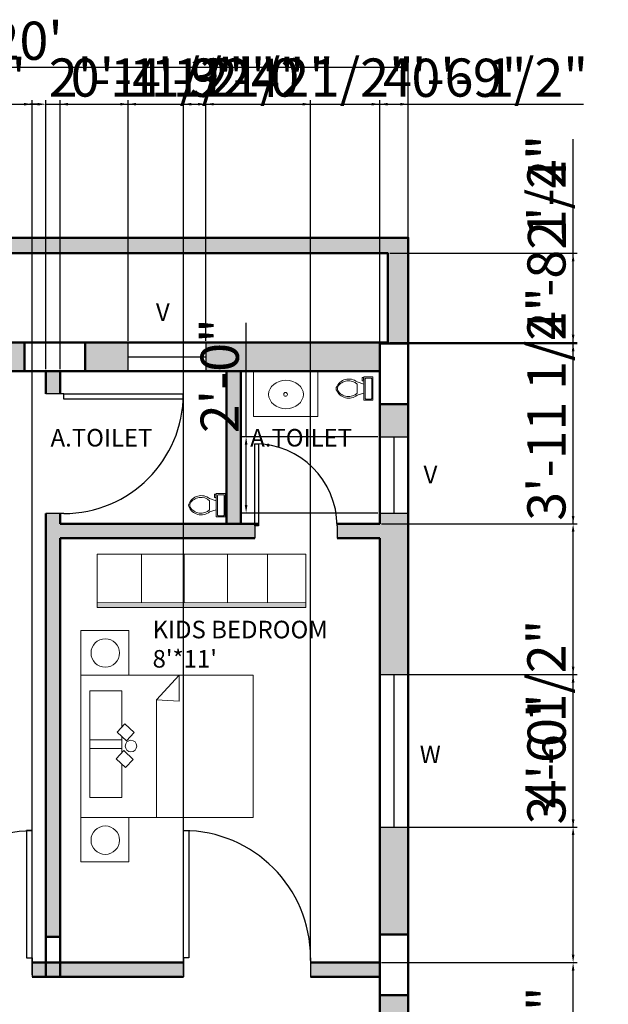
# Model space of a CAD drawing. Units: inches. Extents: x 2063 to 3370, y 2091 to 2971.
# Tile 10 of 14: x 2721 to 2906, y 2623 to 2933. Entities that reach past the tile are written whole.
import ezdxf

# ---------------------------------------------------------------- set-up
doc = ezdxf.new("R2010")
doc.units = ezdxf.units.IN
for name, color, linetype, lineweight in [('A-ANNO-DIMS', 2, 'Continuous', 18), ('A-ANNO-TEXT', 7, 'Continuous', 18), ('A-AREA-IDEN', 3, 'Continuous', 18), ('A-COLS', 7, 'Continuous', 50), ('A-DOOR', 4, 'Continuous', 25), ('A-FLOR-FIXT', 9, 'Continuous', 18), ('A-FURN', 8, 'Continuous', 18), ('A-GLAZ', 131, 'Continuous', 25), ('A-WALL', 7, 'Continuous', 50), ('A-WALL-PATT', 8, 'Continuous', 13)]:
    doc.layers.add(name, color=color, linetype=linetype, lineweight=lineweight)
doc.styles.get("Standard").update_dxf_attribs({"font": 'arial.ttf'})
doc.dimstyles.new('ISO-25', dxfattribs={"dimtxt": 12, "dimasz": 2.5, "dimexe": 1.25, "dimexo": 0.625, "dimtad": 1, "dimdec": 0, "dimlunit": 4, "dimtxsty": 'Standard', "dimcen": 2.5, "dimadec": 0, "dimazin": 0, "dimtfac": 1, "dimtdec": 0, "dimtmove": 0, "dimatfit": 3, "dimfxl": 1, "dimarcsym": 0})

# ---------------------------------------------------------------- blocks, each defined once
blk = doc.blocks.new('*U2')
for p, q in [((0, 0), (0, -6)), ((40, 0), (40, -6))]:
    blk.add_line(p, q)
blk.add_lwpolyline([(0, 0), (0, 40), (1.75, 40), (1.75, 0)], close=True)
blk.add_arc((0, 0), 40, 0, 90)
blk = doc.blocks.new('*U4')
for p, q in [((-10, -8.5), (-8, -8.5)), ((-10, -9.5), (-10, -8.5)), ((-8, -8.5), (-8, -8)), ((-7, -8), (-7, -9.5)), ((-4, -8), (-6, -14)), ((4, -8), (6, -14)), ((9.5, -6), (9.5, -2)), ((-7, -9.5), (-10, -9.5)), ((4, -14), (-4, -14))]:
    blk.add_line(p, q)
blk.add_lwpolyline([(10.5, -8), (10.5, 0), (-10.5, 0), (-10.5, -8)], close=True)
for points in [[(-9.5, -2), (-9.5, -6)], [(8.5, -1), (-8.5, -1)], [(-8.5, -7), (8.5, -7)]]:
    blk.add_lwpolyline(points)
for centre, radius, start, end in [((-8.62, -1.88), 0.884, 81.8699, 188.1301), ((-8.62, -6.12), 0.884, 171.8699, 278.1301), ((8.62, -1.88), 0.884, 351.8699, 98.1301), ((8.62, -6.12), 0.884, 261.8699, 8.1301), ((3.52, -21.58), 12.17, 141.46911, 247.97143), ((4.2, -21.82), 11.33, 136.36773, 238.94682), ((-3.52, -21.58), 12.17, 292.02843, 38.53071), ((-4.2, -21.82), 11.33, 301.05301, 43.63209), ((0, -27.88), 4, 245.73182, 294.26817), ((0, -29), 4, 254.86053, 285.13947)]:
    blk.add_arc(centre, radius, start, end)
blk = doc.blocks.new('*D7')
at = {"layer": 'A-ANNO-DIMS', "color": 0, "lineweight": -2, "transparency": 16777216}
for p, q in [((2602.75, 2865.05), (2602.75, 2919.33)), ((2605.25, 2918.08), (2840.25, 2918.08)), ((2842.75, 2865.05), (2842.75, 2919.33))]:
    blk.add_line(p, q, dxfattribs=at)
at = {"layer": 'A-ANNO-DIMS', "color": 0, "transparency": 16777216}
for points in [[(2605.25, 2918.5), (2605.25, 2917.67), (2602.75, 2918.08)], [(2840.25, 2918.5), (2840.25, 2917.67), (2842.75, 2918.08)]]:
    blk.add_solid(points, dxfattribs=at)
at = {"layer": 'Defpoints', "color": 0, "transparency": 16777216}
for p in [(2842.75, 2918.08), (2602.75, 2864.43), (2842.75, 2864.43)]:
    blk.add_point(p, dxfattribs=at)
at = {"layer": 'A-ANNO-DIMS', "color": 0, "transparency": 16777216, "insert": (2722.75, 2924.84), "char_height": 12, "attachment_point": 5}
blk.add_mtext("20'", dxfattribs=at)
blk = doc.blocks.new('BED-DOUBLE')
for p, q in [((23.79, 50.98), (30.96, 58.78)), ((30.96, 58.78), (30.96, 50.54)), ((23.79, 14), (23.79, 50.98)), ((30.96, 50.54), (23.79, 50.98))]:
    blk.add_line(p, q)
for points in [[(0, 58.78), (15.11, 58.78), (15.11, 72.78), (0, 72.78)], [(0, 58.78), (54.26, 58.78), (54.26, 14), (0, 14)], [(11.45, 40.86), (13.89, 43.46), (16.84, 40.71), (14.4, 38.1)], [(11.16, 32.43), (13.59, 35.03), (16.54, 32.28), (14.11, 29.67)], [(0, 0), (15.11, 0), (15.11, 14), (0, 14)]]:
    blk.add_lwpolyline(points, close=True)
for points in [[(12.88, 42.39), (12.88, 53.87), (2.9, 53.87), (2.9, 35.71), (12.88, 35.71), (12.88, 39.52)], [(12.88, 34.27), (12.88, 38.39), (2.9, 38.39), (2.9, 20.23), (12.88, 20.23), (12.88, 30.81)]]:
    blk.add_lwpolyline(points)
for centre, radius in [((7.71, 65.74), 4.47), ((15.81, 36.46), 1.81), ((7.71, 6.86), 4.47)]:
    blk.add_circle(centre, radius)
blk = doc.blocks.new('WARDROBE')
for p, q in [((13.88, 1.44), (13.88, 16.75)), ((27.33, 1.44), (27.33, 16.75)), ((40.97, 1.44), (40.97, 16.75)), ((53.56, 1.44), (53.56, 16.75)), ((0, 1.42), (65.55, 1.52))]:
    blk.add_line(p, q)
blk.add_lwpolyline([(0, 16.75), (65.55, 16.75), (65.55, 0), (0, 0)], close=True)
blk = doc.blocks.new('*D82')
at = {"layer": 'A-ANNO-DIMS', "color": 0, "lineweight": -2, "transparency": 16777216}
for p, q in [((2703.27, 2832.05), (2703.27, 2907.68)), ((2705.77, 2906.43), (2726.25, 2906.43)), ((2728.75, 2823.05), (2728.75, 2907.68)), ((2728.75, 2906.43), (2792.56, 2906.43))]:
    blk.add_line(p, q, dxfattribs=at)
at = {"layer": 'A-ANNO-DIMS', "color": 0, "transparency": 16777216}
for points in [[(2705.77, 2906.84), (2705.77, 2906.01), (2703.27, 2906.43)], [(2726.25, 2906.84), (2726.25, 2906.01), (2728.75, 2906.43)]]:
    blk.add_solid(points, dxfattribs=at)
at = {"layer": 'Defpoints', "color": 0, "transparency": 16777216}
for p in [(2728.75, 2906.43), (2703.27, 2831.43), (2728.75, 2822.43)]:
    blk.add_point(p, dxfattribs=at)
at = {"layer": 'A-ANNO-DIMS', "color": 0, "transparency": 16777216, "insert": (2761.9, 2913.26), "char_height": 12, "attachment_point": 5}
blk.add_mtext('2\'-1 1/2"', dxfattribs=at)
blk = doc.blocks.new('*D83')
at = {"layer": 'A-ANNO-DIMS', "color": 0, "lineweight": -2, "transparency": 16777216}
for p, q in [((2726.25, 2906.43), (2723.75, 2906.43)), ((2728.75, 2823.05), (2728.75, 2907.68)), ((2728.75, 2906.43), (2733.25, 2906.43)), ((2733.25, 2823.05), (2733.25, 2907.68)), ((2735.75, 2906.43), (2799.36, 2906.43))]:
    blk.add_line(p, q, dxfattribs=at)
at = {"layer": 'A-ANNO-DIMS', "color": 0, "transparency": 16777216}
for points in [[(2726.25, 2906.84), (2726.25, 2906.01), (2728.75, 2906.43)], [(2735.75, 2906.84), (2735.75, 2906.01), (2733.25, 2906.43)]]:
    blk.add_solid(points, dxfattribs=at)
at = {"layer": 'Defpoints', "color": 0, "transparency": 16777216}
for p in [(2733.25, 2906.43), (2728.75, 2822.43), (2733.25, 2822.43)]:
    blk.add_point(p, dxfattribs=at)
at = {"layer": 'A-ANNO-DIMS', "color": 0, "transparency": 16777216, "insert": (2768.8, 2913.26), "char_height": 12, "attachment_point": 5}
blk.add_mtext('0\'-4 1/2"', dxfattribs=at)
blk = doc.blocks.new('*D84')
at = {"layer": 'A-ANNO-DIMS', "color": 0, "lineweight": -2, "transparency": 16777216}
for p, q in [((2733.25, 2823.05), (2733.25, 2907.68)), ((2735.75, 2906.43), (2752.16, 2906.43)), ((2754.66, 2832.05), (2754.66, 2907.68)), ((2754.66, 2906.43), (2817.14, 2906.43))]:
    blk.add_line(p, q, dxfattribs=at)
at = {"layer": 'A-ANNO-DIMS', "color": 0, "transparency": 16777216}
for points in [[(2735.75, 2906.84), (2735.75, 2906.01), (2733.25, 2906.43)], [(2752.16, 2906.84), (2752.16, 2906.01), (2754.66, 2906.43)]]:
    blk.add_solid(points, dxfattribs=at)
at = {"layer": 'Defpoints', "color": 0, "transparency": 16777216}
for p in [(2754.66, 2906.43), (2754.66, 2831.43), (2733.25, 2822.43)]:
    blk.add_point(p, dxfattribs=at)
at = {"layer": 'A-ANNO-DIMS', "color": 0, "transparency": 16777216, "insert": (2787.15, 2913.26), "char_height": 12, "attachment_point": 5}
blk.add_mtext('1\'-9 1/2"', dxfattribs=at)
blk = doc.blocks.new('*D85')
at = {"layer": 'A-ANNO-DIMS', "color": 0, "lineweight": -2, "transparency": 16777216}
for p, q in [((2754.66, 2832.05), (2754.66, 2907.68)), ((2757.16, 2906.43), (2776.59, 2906.43)), ((2779.09, 2832.05), (2779.09, 2907.68)), ((2779.09, 2906.43), (2842.91, 2906.43))]:
    blk.add_line(p, q, dxfattribs=at)
at = {"layer": 'A-ANNO-DIMS', "color": 0, "transparency": 16777216}
for points in [[(2757.16, 2906.84), (2757.16, 2906.01), (2754.66, 2906.43)], [(2776.59, 2906.84), (2776.59, 2906.01), (2779.09, 2906.43)]]:
    blk.add_solid(points, dxfattribs=at)
at = {"layer": 'Defpoints', "color": 0, "transparency": 16777216}
for p in [(2779.09, 2906.43), (2754.66, 2831.43), (2779.09, 2831.43)]:
    blk.add_point(p, dxfattribs=at)
at = {"layer": 'A-ANNO-DIMS', "color": 0, "transparency": 16777216, "insert": (2812.25, 2913.26), "char_height": 12, "attachment_point": 5}
blk.add_mtext('2\'-0 1/2"', dxfattribs=at)
blk = doc.blocks.new('*D86')
at = {"layer": 'A-ANNO-DIMS', "color": 0, "lineweight": -2, "transparency": 16777216}
for p, q in [((2779.09, 2832.05), (2779.09, 2907.68)), ((2781.59, 2906.43), (2831.25, 2906.43)), ((2833.75, 2823.05), (2833.75, 2907.68)), ((2833.75, 2906.43), (2897.84, 2906.43))]:
    blk.add_line(p, q, dxfattribs=at)
at = {"layer": 'A-ANNO-DIMS', "color": 0, "transparency": 16777216}
for points in [[(2781.59, 2906.84), (2781.59, 2906.01), (2779.09, 2906.43)], [(2831.25, 2906.84), (2831.25, 2906.01), (2833.75, 2906.43)]]:
    blk.add_solid(points, dxfattribs=at)
at = {"layer": 'Defpoints', "color": 0, "transparency": 16777216}
for p in [(2833.75, 2906.43), (2779.09, 2831.43), (2833.75, 2822.43)]:
    blk.add_point(p, dxfattribs=at)
at = {"layer": 'A-ANNO-DIMS', "color": 0, "transparency": 16777216, "insert": (2867.04, 2913.26), "char_height": 12, "attachment_point": 5}
blk.add_mtext('4\'-6 1/2"', dxfattribs=at)
blk = doc.blocks.new('*D87')
at = {"layer": 'A-ANNO-DIMS', "color": 0, "lineweight": -2, "transparency": 16777216}
for p, q in [((2833.75, 2823.05), (2833.75, 2907.68)), ((2836.25, 2906.43), (2840.25, 2906.43)), ((2842.75, 2831.77), (2842.75, 2907.68)), ((2842.75, 2906.43), (2878.4, 2906.43))]:
    blk.add_line(p, q, dxfattribs=at)
at = {"layer": 'A-ANNO-DIMS', "color": 0, "transparency": 16777216}
for points in [[(2836.25, 2906.84), (2836.25, 2906.01), (2833.75, 2906.43)], [(2840.25, 2906.84), (2840.25, 2906.01), (2842.75, 2906.43)]]:
    blk.add_solid(points, dxfattribs=at)
at = {"layer": 'Defpoints', "color": 0, "transparency": 16777216}
for p in [(2842.75, 2906.43), (2842.75, 2831.15), (2833.75, 2822.43)]:
    blk.add_point(p, dxfattribs=at)
at = {"layer": 'A-ANNO-DIMS', "color": 0, "transparency": 16777216, "insert": (2861.82, 2913.18), "char_height": 12, "attachment_point": 5}
blk.add_mtext('0\'-9"', dxfattribs=at)
blk = doc.blocks.new('*D119')
at = {"layer": 'A-ANNO-DIMS', "color": 0, "lineweight": -2, "transparency": 16777216}
for p, q in [((2834.37, 2636.43), (2895.82, 2636.43)), ((2894.57, 2587.78), (2894.57, 2633.93)), ((2834.37, 2585.28), (2895.82, 2585.28))]:
    blk.add_line(p, q, dxfattribs=at)
at = {"layer": 'A-ANNO-DIMS', "color": 0, "transparency": 16777216}
for points in [[(2894.15, 2633.93), (2894.99, 2633.93), (2894.57, 2636.43)], [(2894.15, 2587.78), (2894.99, 2587.78), (2894.57, 2585.28)]]:
    blk.add_solid(points, dxfattribs=at)
at = {"layer": 'Defpoints', "color": 0, "transparency": 16777216}
for p in [(2833.75, 2636.43), (2894.57, 2636.43), (2833.75, 2585.28)]:
    blk.add_point(p, dxfattribs=at)
at = {"layer": 'A-ANNO-DIMS', "color": 0, "transparency": 16777216, "insert": (2887.82, 2610.85), "char_height": 12, "attachment_point": 5, "rotation": 90}
blk.add_mtext('4\'-3"', dxfattribs=at)
blk = doc.blocks.new('*D120')
at = {"layer": 'A-ANNO-DIMS', "color": 0, "lineweight": -2, "transparency": 16777216}
for p, q in [((2894.57, 2679.03), (2894.57, 2742.63)), ((2834.37, 2679.03), (2895.82, 2679.03)), ((2894.57, 2638.93), (2894.57, 2676.53)), ((2834.37, 2636.43), (2895.82, 2636.43))]:
    blk.add_line(p, q, dxfattribs=at)
at = {"layer": 'A-ANNO-DIMS', "color": 0, "transparency": 16777216}
for points in [[(2894.15, 2676.53), (2894.99, 2676.53), (2894.57, 2679.03)], [(2894.15, 2638.93), (2894.99, 2638.93), (2894.57, 2636.43)]]:
    blk.add_solid(points, dxfattribs=at)
at = {"layer": 'Defpoints', "color": 0, "transparency": 16777216}
for p in [(2833.75, 2679.03), (2894.57, 2679.03), (2833.75, 2636.43)]:
    blk.add_point(p, dxfattribs=at)
at = {"layer": 'A-ANNO-DIMS', "color": 0, "transparency": 16777216, "insert": (2887.74, 2712.08), "char_height": 12, "attachment_point": 5, "rotation": 90}
blk.add_mtext('3\'-6 1/2"', dxfattribs=at)
blk = doc.blocks.new('*D121')
at = {"layer": 'A-ANNO-DIMS', "color": 0, "lineweight": -2, "transparency": 16777216}
for p, q in [((2834.37, 2727.03), (2895.82, 2727.03)), ((2894.57, 2681.53), (2894.57, 2724.53)), ((2834.37, 2679.03), (2895.82, 2679.03))]:
    blk.add_line(p, q, dxfattribs=at)
at = {"layer": 'A-ANNO-DIMS', "color": 0, "transparency": 16777216}
for points in [[(2894.15, 2724.53), (2894.99, 2724.53), (2894.57, 2727.03)], [(2894.15, 2681.53), (2894.99, 2681.53), (2894.57, 2679.03)]]:
    blk.add_solid(points, dxfattribs=at)
at = {"layer": 'Defpoints', "color": 0, "transparency": 16777216}
for p in [(2833.75, 2727.03), (2894.57, 2727.03), (2833.75, 2679.03)]:
    blk.add_point(p, dxfattribs=at)
at = {"layer": 'A-ANNO-DIMS', "color": 0, "transparency": 16777216, "insert": (2887.82, 2703.03), "char_height": 12, "attachment_point": 5, "rotation": 90}
blk.add_mtext('4\'-0"', dxfattribs=at)
blk = doc.blocks.new('*D122')
at = {"layer": 'A-ANNO-DIMS', "color": 0, "lineweight": -2, "transparency": 16777216}
for p, q in [((2894.57, 2774.43), (2894.57, 2847.35)), ((2834.37, 2774.43), (2895.82, 2774.43)), ((2894.57, 2729.53), (2894.57, 2771.93)), ((2834.37, 2727.03), (2895.82, 2727.03))]:
    blk.add_line(p, q, dxfattribs=at)
at = {"layer": 'A-ANNO-DIMS', "color": 0, "transparency": 16777216}
for points in [[(2894.15, 2771.93), (2894.99, 2771.93), (2894.57, 2774.43)], [(2894.15, 2729.53), (2894.99, 2729.53), (2894.57, 2727.03)]]:
    blk.add_solid(points, dxfattribs=at)
at = {"layer": 'Defpoints', "color": 0, "transparency": 16777216}
for p in [(2833.75, 2774.43), (2894.57, 2774.43), (2833.75, 2727.03)]:
    blk.add_point(p, dxfattribs=at)
at = {"layer": 'A-ANNO-DIMS', "color": 0, "transparency": 16777216, "insert": (2887.74, 2812.14), "char_height": 12, "attachment_point": 5, "rotation": 90}
blk.add_mtext('3\'-11 1/2"', dxfattribs=at)
blk = doc.blocks.new('*D123')
at = {"layer": 'A-ANNO-DIMS', "color": 0, "lineweight": -2, "transparency": 16777216}
for p, q in [((2894.57, 2831.15), (2894.57, 2895.24)), ((2834.37, 2831.15), (2895.82, 2831.15)), ((2894.57, 2776.93), (2894.57, 2828.65)), ((2834.37, 2774.43), (2895.82, 2774.43))]:
    blk.add_line(p, q, dxfattribs=at)
at = {"layer": 'A-ANNO-DIMS', "color": 0, "transparency": 16777216}
for points in [[(2894.15, 2828.65), (2894.99, 2828.65), (2894.57, 2831.15)], [(2894.15, 2776.93), (2894.99, 2776.93), (2894.57, 2774.43)]]:
    blk.add_solid(points, dxfattribs=at)
at = {"layer": 'Defpoints', "color": 0, "transparency": 16777216}
for p in [(2833.75, 2831.15), (2894.57, 2831.15), (2833.75, 2774.43)]:
    blk.add_point(p, dxfattribs=at)
at = {"layer": 'A-ANNO-DIMS', "color": 0, "transparency": 16777216, "insert": (2887.74, 2864.44), "char_height": 12, "attachment_point": 5, "rotation": 90}
blk.add_mtext('4\'-8 1/2"', dxfattribs=at)
blk = doc.blocks.new('*D124')
at = {"layer": 'A-ANNO-DIMS', "color": 0, "lineweight": -2, "transparency": 16777216}
for p, q in [((2894.57, 2859.54), (2894.57, 2895.4)), ((2836.99, 2859.54), (2895.82, 2859.54)), ((2894.57, 2833.93), (2894.57, 2857.04)), ((2836.99, 2831.43), (2895.82, 2831.43))]:
    blk.add_line(p, q, dxfattribs=at)
at = {"layer": 'A-ANNO-DIMS', "color": 0, "transparency": 16777216}
for points in [[(2894.15, 2857.04), (2894.99, 2857.04), (2894.57, 2859.54)], [(2894.15, 2833.93), (2894.99, 2833.93), (2894.57, 2831.43)]]:
    blk.add_solid(points, dxfattribs=at)
at = {"layer": 'Defpoints', "color": 0, "transparency": 16777216}
for p in [(2836.36, 2859.54), (2894.57, 2859.54), (2836.36, 2831.43)]:
    blk.add_point(p, dxfattribs=at)
at = {"layer": 'A-ANNO-DIMS', "color": 0, "transparency": 16777216, "insert": (2887.92, 2878.72), "char_height": 12, "attachment_point": 5, "rotation": 90}
blk.add_mtext('2\'-4"', dxfattribs=at)
blk = doc.blocks.new('*D125')
at = {"layer": 'A-ANNO-DIMS', "color": 0, "lineweight": -2, "transparency": 16777216}
for p, q in [((2791.75, 2801.84), (2791.75, 2837.7)), ((2833.12, 2801.84), (2790.5, 2801.84)), ((2791.75, 2780.34), (2791.75, 2799.34)), ((2833.12, 2777.84), (2790.5, 2777.84))]:
    blk.add_line(p, q, dxfattribs=at)
at = {"layer": 'A-ANNO-DIMS', "color": 0, "transparency": 16777216}
for points in [[(2791.33, 2799.34), (2792.16, 2799.34), (2791.75, 2801.84)], [(2791.33, 2780.34), (2792.16, 2780.34), (2791.75, 2777.84)]]:
    blk.add_solid(points, dxfattribs=at)
at = {"layer": 'Defpoints', "color": 0, "transparency": 16777216}
for p in [(2791.75, 2801.84), (2833.75, 2801.84), (2833.75, 2777.84)]:
    blk.add_point(p, dxfattribs=at)
at = {"layer": 'A-ANNO-DIMS', "color": 0, "transparency": 16777216, "insert": (2785, 2821.02), "char_height": 12, "attachment_point": 5, "rotation": 90}
blk.add_mtext('2\'-0"', dxfattribs=at)
blk = doc.blocks.new('*D128')
at = {"layer": 'A-ANNO-DIMS', "color": 0, "lineweight": -2, "transparency": 16777216}
for p, q in [((2684.44, 2637.05), (2684.44, 2907.68)), ((2686.94, 2906.43), (2721.94, 2906.43)), ((2724.44, 2632.55), (2724.44, 2907.68))]:
    blk.add_line(p, q, dxfattribs=at)
at = {"layer": 'A-ANNO-DIMS', "color": 0, "transparency": 16777216}
for points in [[(2686.94, 2906.84), (2686.94, 2906.01), (2684.44, 2906.43)], [(2721.94, 2906.84), (2721.94, 2906.01), (2724.44, 2906.43)]]:
    blk.add_solid(points, dxfattribs=at)
at = {"layer": 'Defpoints', "color": 0, "transparency": 16777216}
for p in [(2724.44, 2906.43), (2684.44, 2636.43), (2724.44, 2631.93)]:
    blk.add_point(p, dxfattribs=at)
at = {"layer": 'A-ANNO-DIMS', "color": 0, "transparency": 16777216, "insert": (2704.44, 2913.18), "char_height": 12, "attachment_point": 5}
blk.add_mtext('3\'-4"', dxfattribs=at)
blk = doc.blocks.new('*D129')
at = {"layer": 'A-ANNO-DIMS', "color": 0, "lineweight": -2, "transparency": 16777216}
for p, q in [((2772.02, 2632.55), (2772.02, 2907.68)), ((2774.52, 2906.43), (2809.52, 2906.43)), ((2812.02, 2637.05), (2812.02, 2907.68))]:
    blk.add_line(p, q, dxfattribs=at)
at = {"layer": 'A-ANNO-DIMS', "color": 0, "transparency": 16777216}
for points in [[(2774.52, 2906.84), (2774.52, 2906.01), (2772.02, 2906.43)], [(2809.52, 2906.84), (2809.52, 2906.01), (2812.02, 2906.43)]]:
    blk.add_solid(points, dxfattribs=at)
at = {"layer": 'Defpoints', "color": 0, "transparency": 16777216}
for p in [(2812.02, 2906.43), (2812.02, 2636.43), (2772.02, 2631.93)]:
    blk.add_point(p, dxfattribs=at)
at = {"layer": 'A-ANNO-DIMS', "color": 0, "transparency": 16777216, "insert": (2792.02, 2913.18), "char_height": 12, "attachment_point": 5}
blk.add_mtext('3\'-4"', dxfattribs=at)

msp = doc.modelspace()

# ---------------------------------------------------------------- hatches: boundary and pattern name
at = {"layer": 'A-FURN'}
h = msp.add_hatch(color=256, dxfattribs=at)
h.dxf.hatch_style = 1
h.paths.add_polyline_path([(2810.49, 2749.65), (2744.95, 2749.56), (2744.95, 2748.13), (2810.49, 2748.13)])
at = {"layer": 'A-WALL-PATT'}
h = msp.add_hatch(color=256, dxfattribs=at)
h.dxf.hatch_style = 1
h.paths.add_polyline_path([(2842.75, 2864.43), (2602.75, 2864.43), (2602.75, 2831.43), (2608.62, 2831.43), (2608.62, 2859.54), (2836.36, 2859.54), (2836.36, 2831.15), (2842.75, 2831.15)])
h.paths.add_polyline_path([(2775.49, 2177.04), (2815.13, 2177.04), (2815.13, 2197.65), (2775.49, 2197.65)], flags=9)
h.paths.add_polyline_path([(2634.18, 2285.75), (2670.81, 2285.75), (2670.81, 2306.35), (2634.18, 2306.35)], flags=9)
h.paths.add_polyline_path([(2701.65, 2293.1), (2755.85, 2293.1), (2755.85, 2313.71), (2701.65, 2313.71)], flags=9)
h.paths.add_polyline_path([(2735.8, 2415.55), (2772.95, 2415.55), (2772.95, 2436.13), (2735.8, 2436.13)], flags=9)
h.paths.add_polyline_path([(2641.75, 2422.21), (2718.67, 2422.21), (2718.67, 2442.82), (2641.75, 2442.82)], flags=9)
h.paths.add_polyline_path([(2710.43, 2552.92), (2764.91, 2552.92), (2764.91, 2573.53), (2710.43, 2573.53)], flags=9)
h.paths.add_polyline_path([(2625.23, 2527.83), (2661.86, 2527.83), (2661.86, 2548.44), (2625.23, 2548.44)], flags=9)
h.paths.add_polyline_path([(2627.53, 2598.16), (2652.13, 2598.16), (2652.13, 2618.77), (2627.53, 2618.77)], flags=9)
h.paths.add_polyline_path([(2646.64, 2696.08), (2723.56, 2696.08), (2723.56, 2716.69), (2646.64, 2716.69)], flags=9)
h.paths.add_polyline_path([(2791.65, 2795.64), (2828.72, 2795.64), (2828.72, 2807.02), (2791.65, 2807.02)], flags=9)
h.paths.add_polyline_path([(2751.88, 2214.78), (2761.93, 2214.78), (2761.93, 2226.17), (2751.88, 2226.17)], flags=9)
h.paths.add_polyline_path([(2664.96, 2215.71), (2675, 2215.71), (2675, 2227.09), (2664.96, 2227.09)], flags=9)
h.paths.add_polyline_path([(2788.26, 2413.43), (2796.17, 2413.43), (2796.17, 2424.82), (2788.26, 2424.82)], flags=9)
h.paths.add_polyline_path([(2728.86, 2795.64), (2765.93, 2795.64), (2765.93, 2807.02), (2728.86, 2807.02)], flags=9)
h.paths.add_polyline_path([(2760.39, 2726.09), (2823.16, 2726.09), (2823.16, 2746.7), (2760.39, 2746.7)], flags=9)
h = msp.add_hatch(color=256, dxfattribs=at)
h.dxf.hatch_style = 1
h.paths.add_polyline_path([(2290.22, 2192.43), (2278.22, 2192.43), (2182.22, 2192.43), (2182.22, 2189.43), (2182.22, 2187.43), (2278.22, 2187.43), (2290.22, 2187.42)])
h.paths.add_polyline_path([(2748.25, 2192.43), (2736.25, 2192.43), (2640.25, 2192.43), (2640.25, 2189.43), (2640.25, 2187.43), (2736.25, 2187.43), (2748.25, 2187.42)], flags=17)
h.paths.add_polyline_path([(2653.66, 2234.43), (2611.75, 2234.43), (2611.75, 2232.93), (2611.75, 2225.43), (2653.66, 2225.43)])
h.paths.add_polyline_path([(2717.13, 2234.43), (2675.81, 2234.43), (2675.81, 2225.43), (2717.13, 2225.43)])
h.paths.add_polyline_path([(2611.75, 2222.57), (2602.75, 2222.57), (2602.75, 2144.43), (2842.75, 2144.43), (2842.75, 2220.3), (2833.75, 2220.3), (2833.75, 2153.43), (2829.39, 2153.43), (2754.78, 2153.43), (2611.75, 2153.43)])
h.paths.add_polyline_path([(2687.64, 2308.91), (2683.14, 2308.91), (2683.14, 2234.43), (2687.64, 2234.43)])
h.paths.add_polyline_path([(2744.5, 2234.43), (2736.25, 2234.43), (2736.25, 2225.43), (2744.5, 2225.43)])
h.paths.add_polyline_path([(2785.14, 2260.02), (2782.31, 2260.02), (2780.64, 2260.02), (2780.64, 2234.43), (2766.65, 2234.43), (2766.65, 2225.43), (2785.14, 2225.43)])
h.paths.add_polyline_path([(2842.75, 2363.93), (2833.75, 2363.93), (2833.75, 2239.41), (2842.75, 2239.41)])
h.paths.add_polyline_path([(2775.49, 2177.04), (2815.13, 2177.04), (2815.13, 2197.65), (2775.49, 2197.65)], flags=25)
h.paths.add_polyline_path([(2634.18, 2285.75), (2670.81, 2285.75), (2670.81, 2306.35), (2634.18, 2306.35)], flags=9)
h.paths.add_polyline_path([(2701.65, 2293.1), (2755.85, 2293.1), (2755.85, 2313.71), (2701.65, 2313.71)], flags=9)
h.paths.add_polyline_path([(2735.8, 2415.55), (2772.95, 2415.55), (2772.95, 2436.13), (2735.8, 2436.13)], flags=9)
h.paths.add_polyline_path([(2641.75, 2422.21), (2718.67, 2422.21), (2718.67, 2442.82), (2641.75, 2442.82)], flags=9)
h.paths.add_polyline_path([(2710.43, 2552.92), (2764.91, 2552.92), (2764.91, 2573.53), (2710.43, 2573.53)], flags=9)
h.paths.add_polyline_path([(2625.23, 2527.83), (2661.86, 2527.83), (2661.86, 2548.44), (2625.23, 2548.44)], flags=9)
h.paths.add_polyline_path([(2627.53, 2598.16), (2652.13, 2598.16), (2652.13, 2618.77), (2627.53, 2618.77)], flags=9)
h.paths.add_polyline_path([(2646.64, 2696.08), (2723.56, 2696.08), (2723.56, 2716.69), (2646.64, 2716.69)], flags=9)
h.paths.add_polyline_path([(2791.65, 2795.64), (2828.72, 2795.64), (2828.72, 2807.02), (2791.65, 2807.02)], flags=9)
h.paths.add_polyline_path([(2751.88, 2214.78), (2761.93, 2214.78), (2761.93, 2226.17), (2751.88, 2226.17)], flags=9)
h.paths.add_polyline_path([(2788.26, 2413.43), (2796.17, 2413.43), (2796.17, 2424.82), (2788.26, 2424.82)], flags=9)
h.paths.add_polyline_path([(2761.97, 2835.24), (2769.88, 2835.24), (2769.88, 2846.62), (2761.97, 2846.62)], flags=9)
h.paths.add_polyline_path([(2675.89, 2833.68), (2685.93, 2833.68), (2685.93, 2845.06), (2675.89, 2845.06)], flags=9)
h.paths.add_polyline_path([(2728.86, 2795.64), (2765.93, 2795.64), (2765.93, 2807.02), (2728.86, 2807.02)], flags=9)
h.paths.add_polyline_path([(2760.39, 2726.09), (2823.16, 2726.09), (2823.16, 2746.7), (2760.39, 2746.7)], flags=9)
h = msp.add_hatch(color=256, dxfattribs=at)
h.dxf.hatch_style = 1
h.paths.add_polyline_path([(2680.75, 2631.93), (2684.44, 2631.93), (2684.44, 2636.43), (2683.1, 2636.43), (2611.75, 2636.43), (2611.75, 2631.93), (2648.72, 2631.93), (2671.75, 2631.93), (2676.25, 2631.93), (2676.25, 2623.58), (2678.23, 2623.58), (2680.75, 2623.58)])
h.paths.add_polyline_path([(2728.75, 2636.43), (2724.44, 2636.43), (2724.44, 2631.93), (2728.75, 2631.93)])
h.paths.add_polyline_path([(2772.02, 2636.43), (2733.25, 2636.43), (2733.25, 2631.93), (2772.02, 2631.93)])
h.paths.add_polyline_path([(2733.25, 2636.43), (2728.75, 2636.43), (2728.75, 2631.93), (2733.25, 2631.93)])
h.paths.add_polyline_path([(2833.75, 2636.43), (2812.02, 2636.43), (2812.02, 2631.93), (2833.75, 2631.93)])
h.paths.add_polyline_path([(2842.75, 2626.16), (2833.75, 2626.16), (2833.75, 2585.28), (2842.75, 2585.28)])
h.paths.add_polyline_path([(2842.75, 2679.03), (2833.75, 2679.03), (2833.75, 2645.28), (2842.75, 2645.28)])
h.paths.add_polyline_path([(2611.75, 2619.52), (2602.75, 2619.52), (2602.75, 2548.5), (2611.75, 2548.5), (2611.75, 2579.43)])
h.paths.add_polyline_path([(2646.64, 2696.08), (2723.56, 2696.08), (2723.56, 2716.69), (2646.64, 2716.69)], flags=9)
h.paths.add_polyline_path([(2791.65, 2795.64), (2828.72, 2795.64), (2828.72, 2807.02), (2791.65, 2807.02)], flags=9)
h.paths.add_polyline_path([(2761.97, 2835.24), (2769.88, 2835.24), (2769.88, 2846.62), (2761.97, 2846.62)], flags=9)
h.paths.add_polyline_path([(2675.89, 2833.68), (2685.93, 2833.68), (2685.93, 2845.06), (2675.89, 2845.06)], flags=9)
h.paths.add_polyline_path([(2728.86, 2795.64), (2765.93, 2795.64), (2765.93, 2807.02), (2728.86, 2807.02)], flags=9)
h.paths.add_polyline_path([(2775.49, 2177.04), (2815.13, 2177.04), (2815.13, 2197.65), (2775.49, 2197.65)], flags=9)
h.paths.add_polyline_path([(2634.18, 2285.75), (2670.81, 2285.75), (2670.81, 2306.35), (2634.18, 2306.35)], flags=9)
h.paths.add_polyline_path([(2701.65, 2293.1), (2755.85, 2293.1), (2755.85, 2313.71), (2701.65, 2313.71)], flags=9)
h.paths.add_polyline_path([(2735.8, 2415.55), (2772.95, 2415.55), (2772.95, 2436.13), (2735.8, 2436.13)], flags=9)
h.paths.add_polyline_path([(2641.75, 2422.21), (2718.67, 2422.21), (2718.67, 2442.82), (2641.75, 2442.82)], flags=9)
h.paths.add_polyline_path([(2710.43, 2552.92), (2764.91, 2552.92), (2764.91, 2573.53), (2710.43, 2573.53)], flags=9)
h.paths.add_polyline_path([(2625.23, 2527.83), (2661.86, 2527.83), (2661.86, 2548.44), (2625.23, 2548.44)], flags=9)
h.paths.add_polyline_path([(2751.88, 2214.78), (2761.93, 2214.78), (2761.93, 2226.17), (2751.88, 2226.17)], flags=9)
h.paths.add_polyline_path([(2664.96, 2215.71), (2675, 2215.71), (2675, 2227.09), (2664.96, 2227.09)], flags=9)
h.paths.add_polyline_path([(2788.26, 2413.43), (2796.17, 2413.43), (2796.17, 2424.82), (2788.26, 2424.82)], flags=9)
h = msp.add_hatch(color=256, dxfattribs=at)
h.dxf.hatch_style = 1
h.paths.add_polyline_path([(2611.75, 2343.93), (2611.75, 2477.43), (2611.75, 2514.15), (2602.75, 2514.15), (2602.75, 2241.68), (2611.75, 2241.68), (2611.75, 2258.43)])
h.paths.add_polyline_path([(2775.49, 2177.04), (2815.13, 2177.04), (2815.13, 2197.65), (2775.49, 2197.65)], flags=9)
h.paths.add_polyline_path([(2735.8, 2415.55), (2772.95, 2415.55), (2772.95, 2436.13), (2735.8, 2436.13)], flags=9)
h.paths.add_polyline_path([(2641.75, 2422.21), (2718.67, 2422.21), (2718.67, 2442.82), (2641.75, 2442.82)], flags=9)
h.paths.add_polyline_path([(2710.43, 2552.92), (2764.91, 2552.92), (2764.91, 2573.53), (2710.43, 2573.53)], flags=9)
h.paths.add_polyline_path([(2625.23, 2527.83), (2661.86, 2527.83), (2661.86, 2548.44), (2625.23, 2548.44)], flags=9)
h.paths.add_polyline_path([(2627.53, 2598.16), (2652.13, 2598.16), (2652.13, 2618.77), (2627.53, 2618.77)], flags=9)
h.paths.add_polyline_path([(2646.64, 2696.08), (2723.56, 2696.08), (2723.56, 2716.69), (2646.64, 2716.69)], flags=9)
h.paths.add_polyline_path([(2791.65, 2795.64), (2828.72, 2795.64), (2828.72, 2807.02), (2791.65, 2807.02)], flags=9)
h.paths.add_polyline_path([(2751.88, 2214.78), (2761.93, 2214.78), (2761.93, 2226.17), (2751.88, 2226.17)], flags=9)
h.paths.add_polyline_path([(2788.26, 2413.43), (2796.17, 2413.43), (2796.17, 2424.82), (2788.26, 2424.82)], flags=9)
h.paths.add_polyline_path([(2761.97, 2835.24), (2769.88, 2835.24), (2769.88, 2846.62), (2761.97, 2846.62)], flags=9)
h.paths.add_polyline_path([(2675.89, 2833.68), (2685.93, 2833.68), (2685.93, 2845.06), (2675.89, 2845.06)], flags=9)
h.paths.add_polyline_path([(2728.86, 2795.64), (2765.93, 2795.64), (2765.93, 2807.02), (2728.86, 2807.02)], flags=9)
h.paths.add_polyline_path([(2760.39, 2726.09), (2823.16, 2726.09), (2823.16, 2746.7), (2760.39, 2746.7)], flags=9)
h = msp.add_hatch(color=256, dxfattribs=at)
h.dxf.hatch_style = 1
h.paths.add_polyline_path([(2785.14, 2468.43), (2780.64, 2468.43), (2780.64, 2429.31), (2785.14, 2429.31)])
h.paths.add_polyline_path([(2842.75, 2525.28), (2833.75, 2525.28), (2833.75, 2523.93), (2833.75, 2466.93), (2833.75, 2383.04), (2842.75, 2383.04)])
h.paths.add_polyline_path([(2789.73, 2477.43), (2680.75, 2477.43), (2680.75, 2579.43), (2680.75, 2589.96), (2678.23, 2589.96), (2676.25, 2589.96), (2676.25, 2583.93), (2667.25, 2583.93), (2611.75, 2583.93), (2611.75, 2579.43), (2671.75, 2579.43), (2676.25, 2579.43), (2676.25, 2477.43), (2611.75, 2477.43), (2611.75, 2468.43), (2728.75, 2468.43), (2789.73, 2468.43), (2789.73, 2471.41)])
h.paths.add_polyline_path([(2710.43, 2552.92), (2764.91, 2552.92), (2764.91, 2573.53), (2710.43, 2573.53)], flags=25)
h.paths.add_polyline_path([(2625.23, 2527.83), (2661.86, 2527.83), (2661.86, 2548.44), (2625.23, 2548.44)], flags=25)
h.paths.add_polyline_path([(2627.53, 2598.16), (2652.13, 2598.16), (2652.13, 2618.77), (2627.53, 2618.77)], flags=9)
h.paths.add_polyline_path([(2646.64, 2696.08), (2723.56, 2696.08), (2723.56, 2716.69), (2646.64, 2716.69)], flags=9)
h.paths.add_polyline_path([(2791.65, 2795.64), (2828.72, 2795.64), (2828.72, 2807.02), (2791.65, 2807.02)], flags=9)
h.paths.add_polyline_path([(2761.97, 2835.24), (2769.88, 2835.24), (2769.88, 2846.62), (2761.97, 2846.62)], flags=9)
h.paths.add_polyline_path([(2675.89, 2833.68), (2685.93, 2833.68), (2685.93, 2845.06), (2675.89, 2845.06)], flags=9)
h.paths.add_polyline_path([(2728.86, 2795.64), (2765.93, 2795.64), (2765.93, 2807.02), (2728.86, 2807.02)], flags=9)
h.paths.add_polyline_path([(2760.39, 2726.09), (2823.16, 2726.09), (2823.16, 2746.7), (2760.39, 2746.7)], flags=9)
h.paths.add_polyline_path([(2775.49, 2177.04), (2815.13, 2177.04), (2815.13, 2197.65), (2775.49, 2197.65)], flags=9)
h.paths.add_polyline_path([(2634.18, 2285.75), (2670.81, 2285.75), (2670.81, 2306.35), (2634.18, 2306.35)], flags=9)
h.paths.add_polyline_path([(2701.65, 2293.1), (2755.85, 2293.1), (2755.85, 2313.71), (2701.65, 2313.71)], flags=9)
h.paths.add_polyline_path([(2641.75, 2422.21), (2718.67, 2422.21), (2718.67, 2442.82), (2641.75, 2442.82)], flags=9)
h.paths.add_polyline_path([(2751.88, 2214.78), (2761.93, 2214.78), (2761.93, 2226.17), (2751.88, 2226.17)], flags=9)
h.paths.add_polyline_path([(2664.96, 2215.71), (2675, 2215.71), (2675, 2227.09), (2664.96, 2227.09)], flags=9)
h.paths.add_polyline_path([(2788.26, 2413.43), (2796.17, 2413.43), (2796.17, 2424.82), (2788.26, 2424.82)], flags=9)
h = msp.add_hatch(color=256, dxfattribs=at)
h.dxf.hatch_style = 1
h.paths.add_polyline_path([(2785.14, 2343.93), (2785.14, 2392.49), (2785.14, 2413.72), (2780.64, 2413.72), (2780.64, 2384.43), (2780.64, 2348.43), (2732.64, 2348.43), (2732.64, 2360.22), (2728.14, 2360.22), (2728.14, 2348.43), (2725.61, 2348.43), (2725.61, 2348.17), (2725.61, 2343.93), (2780.64, 2343.93), (2780.64, 2329.91), (2780.64, 2297.78), (2782.31, 2297.78), (2785.14, 2297.78)])
h.paths.add_polyline_path([(2732.64, 2396.29), (2731.36, 2396.29), (2728.14, 2396.29), (2728.14, 2379.34), (2732.64, 2379.34)], flags=17)
h.paths.add_polyline_path([(2732.64, 2468.43), (2728.14, 2468.43), (2728.14, 2417.8), (2731.36, 2417.8, -0.014809), (2732.64, 2417.76)])
h.paths.add_polyline_path([(2697.29, 2348.43), (2611.75, 2348.43), (2611.75, 2343.93), (2683.14, 2343.93), (2697.29, 2343.93)])
h.paths.add_polyline_path([(2710.43, 2552.92), (2764.91, 2552.92), (2764.91, 2573.53), (2710.43, 2573.53)], flags=9)
h.paths.add_polyline_path([(2625.23, 2527.83), (2661.86, 2527.83), (2661.86, 2548.44), (2625.23, 2548.44)], flags=9)
h.paths.add_polyline_path([(2627.53, 2598.16), (2652.13, 2598.16), (2652.13, 2618.77), (2627.53, 2618.77)], flags=9)
h.paths.add_polyline_path([(2646.64, 2696.08), (2723.56, 2696.08), (2723.56, 2716.69), (2646.64, 2716.69)], flags=9)
h.paths.add_polyline_path([(2791.65, 2795.64), (2828.72, 2795.64), (2828.72, 2807.02), (2791.65, 2807.02)], flags=9)
h.paths.add_polyline_path([(2761.97, 2835.24), (2769.88, 2835.24), (2769.88, 2846.62), (2761.97, 2846.62)], flags=9)
h.paths.add_polyline_path([(2675.89, 2833.68), (2685.93, 2833.68), (2685.93, 2845.06), (2675.89, 2845.06)], flags=9)
h.paths.add_polyline_path([(2728.86, 2795.64), (2765.93, 2795.64), (2765.93, 2807.02), (2728.86, 2807.02)], flags=9)
h.paths.add_polyline_path([(2760.39, 2726.09), (2823.16, 2726.09), (2823.16, 2746.7), (2760.39, 2746.7)], flags=9)
h = msp.add_hatch(color=256, dxfattribs=at)
h.dxf.hatch_style = 1
h.paths.add_polyline_path([(2655.27, 2831.43), (2611.75, 2831.43), (2611.75, 2822.43), (2655.27, 2822.43)])
h.paths.add_polyline_path([(2722.06, 2831.43), (2703.27, 2831.43), (2703.27, 2822.43), (2722.06, 2822.43)])
h.paths.add_polyline_path([(2754.66, 2831.43), (2741.18, 2831.43), (2741.18, 2822.43), (2754.66, 2822.43)])
h.paths.add_polyline_path([(2833.75, 2831.43), (2779.09, 2831.43), (2779.09, 2822.43), (2833.75, 2822.43)])
h.paths.add_polyline_path([(2790.07, 2822.43), (2785.57, 2822.43), (2785.57, 2774.43), (2790.07, 2774.43)])
h.paths.add_polyline_path([(2775.49, 2177.04), (2815.13, 2177.04), (2815.13, 2197.65), (2775.49, 2197.65)], flags=9)
h.paths.add_polyline_path([(2634.18, 2285.75), (2670.81, 2285.75), (2670.81, 2306.35), (2634.18, 2306.35)], flags=9)
h.paths.add_polyline_path([(2701.65, 2293.1), (2755.85, 2293.1), (2755.85, 2313.71), (2701.65, 2313.71)], flags=9)
h.paths.add_polyline_path([(2735.8, 2415.55), (2772.95, 2415.55), (2772.95, 2436.13), (2735.8, 2436.13)], flags=9)
h.paths.add_polyline_path([(2641.75, 2422.21), (2718.67, 2422.21), (2718.67, 2442.82), (2641.75, 2442.82)], flags=9)
h.paths.add_polyline_path([(2710.43, 2552.92), (2764.91, 2552.92), (2764.91, 2573.53), (2710.43, 2573.53)], flags=9)
h.paths.add_polyline_path([(2625.23, 2527.83), (2661.86, 2527.83), (2661.86, 2548.44), (2625.23, 2548.44)], flags=9)
h.paths.add_polyline_path([(2627.53, 2598.16), (2652.13, 2598.16), (2652.13, 2618.77), (2627.53, 2618.77)], flags=9)
h.paths.add_polyline_path([(2646.64, 2696.08), (2723.56, 2696.08), (2723.56, 2716.69), (2646.64, 2716.69)], flags=9)
h.paths.add_polyline_path([(2791.65, 2795.64), (2828.72, 2795.64), (2828.72, 2807.02), (2791.65, 2807.02)], flags=9)
h.paths.add_polyline_path([(2751.88, 2214.78), (2761.93, 2214.78), (2761.93, 2226.17), (2751.88, 2226.17)], flags=9)
h.paths.add_polyline_path([(2664.96, 2215.71), (2675, 2215.71), (2675, 2227.09), (2664.96, 2227.09)], flags=9)
h.paths.add_polyline_path([(2788.26, 2413.43), (2796.17, 2413.43), (2796.17, 2424.82), (2788.26, 2424.82)], flags=9)
h.paths.add_polyline_path([(2728.86, 2795.64), (2765.93, 2795.64), (2765.93, 2807.02), (2728.86, 2807.02)], flags=9)
h.paths.add_polyline_path([(2760.39, 2726.09), (2823.16, 2726.09), (2823.16, 2746.7), (2760.39, 2746.7)], flags=9)
h = msp.add_hatch(color=256, dxfattribs=at)
h.dxf.hatch_style = 1
h.paths.add_polyline_path([(2733.25, 2822.43), (2728.75, 2822.43), (2728.75, 2815.29), (2733.25, 2815.29)])
h.paths.add_polyline_path([(2842.75, 2812.03), (2833.75, 2812.03), (2833.75, 2801.84), (2842.75, 2801.84)])
edge = h.paths.add_edge_path()
edge.add_arc((2794.51, 2773.8), 25.82, 0, 1.391)
edge.add_line((2820.32, 2774.43), (2833.75, 2774.43))
edge.add_line((2833.75, 2774.43), (2833.75, 2777.84))
edge.add_line((2833.75, 2777.84), (2842.75, 2777.84))
edge.add_line((2842.75, 2777.84), (2842.75, 2727.03))
edge.add_line((2842.75, 2727.03), (2833.75, 2727.03))
edge.add_line((2833.75, 2727.03), (2833.75, 2769.93))
edge.add_line((2833.75, 2769.93), (2820.33, 2769.93))
edge.add_line((2820.33, 2769.93), (2820.33, 2773.8))
h.paths.add_polyline_path([(2794.51, 2769.93), (2794.51, 2774.43), (2733.25, 2774.43), (2733.25, 2777.68), (2728.75, 2777.68), (2728.75, 2644.58), (2733.25, 2644.58), (2733.25, 2769.93)])

# ---------------------------------------------------------------- linework, layer by layer
at = {"layer": 'A-COLS'}
for points in [[(2722.06, 2822.43), (2722.06, 2831.43), (2741.18, 2831.43), (2741.18, 2822.43)], [(2833.75, 2831.15), (2842.75, 2831.15), (2842.75, 2812.03), (2833.75, 2812.03)]]:
    msp.add_lwpolyline(points, close=True, dxfattribs=at)
msp.add_lwpolyline([(2833.75, 2636.43), (2833.75, 2645.28), (2842.75, 2645.28), (2842.75, 2626.16), (2833.75, 2626.16), (2833.75, 2631.93)], dxfattribs=at)
at = {"layer": 'A-FLOR-FIXT'}
msp.add_lwpolyline([(2794.04, 2808.22), (2814.32, 2808.22), (2814.32, 2822.43), (2794.04, 2822.43)], close=True, dxfattribs=at)
msp.add_circle((2804.16, 2815.16), 0.596, dxfattribs=at)
msp.add_ellipse((2804.29, 2815.13), major_axis=(5.46, 0), ratio=0.818182, dxfattribs=at)
at = {"layer": 'A-GLAZ'}
for p, q in [((2754.66, 2826.93), (2779.09, 2826.93)), ((2833.75, 2801.84), (2842.75, 2801.84)), ((2838.25, 2801.84), (2838.25, 2777.84)), ((2833.75, 2777.84), (2842.75, 2777.84)), ((2833.75, 2727.03), (2842.75, 2727.03)), ((2838.25, 2727.03), (2838.25, 2679.03)), ((2833.75, 2679.03), (2842.75, 2679.03))]:
    msp.add_line(p, q, dxfattribs=at)
msp.add_lwpolyline([(2754.66, 2831.43), (2779.09, 2831.43), (2779.09, 2822.43), (2754.66, 2822.43)], close=True, dxfattribs=at)
at = {"layer": 'A-WALL'}
for p, q in [((2611.75, 2822.43), (2728.75, 2822.43)), ((2611.75, 2822.43), (2728.75, 2822.43)), ((2728.75, 2822.43), (2728.75, 2815.29)), ((2733.25, 2822.43), (2833.75, 2822.43)), ((2733.25, 2822.43), (2733.25, 2815.29)), ((2733.25, 2822.43), (2733.25, 2815.29)), ((2785.57, 2822.43), (2785.57, 2774.43)), ((2790.07, 2822.43), (2790.07, 2774.43)), ((2728.75, 2777.68), (2728.75, 2631.93)), ((2733.25, 2777.68), (2733.25, 2774.43)), ((2733.25, 2777.68), (2733.25, 2774.43)), ((2733.25, 2774.43), (2795.64, 2774.43)), ((2820.32, 2774.43), (2833.75, 2774.43)), ((2829.25, 2774.43), (2833.75, 2774.43)), ((2733.25, 2769.93), (2733.25, 2631.93)), ((2733.25, 2769.93), (2794.51, 2769.93)), ((2820.33, 2769.93), (2833.75, 2769.93)), ((2724.44, 2636.43), (2772.02, 2636.43)), ((2812.02, 2636.43), (2833.75, 2636.43)), ((2724.44, 2631.93), (2772.02, 2631.93)), ((2812.02, 2631.93), (2833.75, 2631.93))]:
    msp.add_line(p, q, dxfattribs=at)
for points in [[(2602.75, 2144.43), (2842.75, 2144.43), (2842.75, 2864.43), (2602.75, 2864.43)], [(2836.36, 2831.43), (2836.36, 2859.54), (2608.62, 2859.54), (2608.62, 2831.43)]]:
    msp.add_lwpolyline(points, close=True, dxfattribs=at)
for points in [[(2833.75, 2774.43), (2833.75, 2822.43)], [(2833.75, 2576.43), (2833.75, 2769.93)], [(2728.75, 2644.58), (2733.25, 2644.58), (2733.25, 2631.93)]]:
    msp.add_lwpolyline(points, dxfattribs=at)

# ---------------------------------------------------------------- block references
at = {"layer": 'A-DOOR', "xscale": 0.9400530028669262, "yscale": 0.9400530028669262, "zscale": 0.9400530028669262, "rotation": 270}
msp.add_blockref('*U2', (2734.39, 2815.29), dxfattribs=at)
at = {"layer": 'A-DOOR', "xscale": 0.645531349072257, "yscale": 0.645531349072257, "zscale": 0.645531349072257}
msp.add_blockref('*U2', (2794.51, 2773.8), dxfattribs=at)
at = {"layer": 'A-DOOR', "xscale": -1}
msp.add_blockref('*U2', (2724.44, 2637.93), dxfattribs=at)
at = {"layer": 'A-DOOR'}
msp.add_blockref('*U2', (2772.02, 2637.93), dxfattribs=at)
at = {"layer": 'A-FLOR-FIXT', "xscale": 0.3494779928887701, "yscale": 0.3494779928887701, "zscale": 0.3494779928887701, "rotation": 270}
for p in [(2831.6, 2816.96), (2785.17, 2780.28)]:
    msp.add_blockref('*U4', p, dxfattribs=at)
at = {"layer": 'A-FURN'}
for name, p in [('WARDROBE', (2744.95, 2748.13)), ('BED-DOUBLE', (2739.74, 2668.08))]:
    msp.add_blockref(name, p, dxfattribs=at)

# ---------------------------------------------------------------- texts
at = {"layer": 'A-ANNO-TEXT', "char_height": 5.52, "attachment_point": 1}
for s, insert in [('V', (2763.39, 2843.78)), ('V', (2847.55, 2792.69)), ('W', (2846.35, 2704.68))]:
    msp.add_mtext_dynamic_manual_height_columns(s, width=106.0361, gutter_width=27.61, heights=[0], dxfattribs=dict(at, insert=insert))
at = {"layer": 'A-AREA-IDEN', "attachment_point": 1}
for s, insert, char_height in [('A.TOILET', (2730.26, 2804.28), 5.523), ('A.TOILET', (2793.04, 2804.28), 5.523), ("KIDS BEDROOM\\P8'*11'", (2762.33, 2743.95), 5.5229)]:
    msp.add_mtext_dynamic_manual_height_columns(s, width=106.0361, gutter_width=27.61, heights=[0], dxfattribs=dict(at, insert=insert, char_height=char_height))

# ---------------------------------------------------------------- dimensions: what is measured, and where the dimension line sits
at = {"layer": 'A-ANNO-DIMS'}
for base, p1, p2, override, picture, middle in [((2842.75, 2918.08), (2602.75, 2864.43), (2842.75, 2864.43), {"dimclrd": 0, "dimclre": 0, "dimclrt": 0}, '*D7', (2722.75, 2924.84)), ((2728.75, 2906.43), (2703.27, 2831.43), (2728.75, 2822.43), {"dimdec": 1, "dimlfac": 1, "dimrnd": 0, "dimzin": 1, "dimdsep": 46, "dimlunit": 4, "dimfrac": 2}, '*D82', (2761.9, 2913.26)), ((2733.25, 2906.43), (2728.75, 2822.43), (2733.25, 2822.43), {"dimdec": 1, "dimlfac": 1, "dimrnd": 0, "dimzin": 1, "dimdsep": 46, "dimlunit": 4, "dimfrac": 2}, '*D83', (2768.8, 2913.26)), ((2754.66, 2906.43), (2733.25, 2822.43), (2754.66, 2831.43), {"dimdec": 1, "dimlfac": 1, "dimrnd": 0, "dimzin": 1, "dimdsep": 46, "dimlunit": 4, "dimfrac": 2}, '*D84', (2787.15, 2913.26)), ((2779.09, 2906.43), (2754.66, 2831.43), (2779.09, 2831.43), {"dimdec": 1, "dimlfac": 1, "dimrnd": 0, "dimzin": 1, "dimdsep": 46, "dimlunit": 4, "dimfrac": 2}, '*D85', (2812.25, 2913.26)), ((2833.75, 2906.43), (2779.09, 2831.43), (2833.75, 2822.43), {"dimdec": 1, "dimlfac": 1, "dimrnd": 0, "dimzin": 1, "dimdsep": 46, "dimlunit": 4, "dimfrac": 2}, '*D86', (2867.04, 2913.26)), ((2724.44, 2906.43), (2684.44, 2636.43), (2724.44, 2631.93), {"dimdec": 1, "dimlfac": 1, "dimrnd": 0, "dimzin": 1, "dimdsep": 46, "dimlunit": 4, "dimfrac": 2}, '*D128', (2704.44, 2913.18)), ((2812.02, 2906.43), (2772.02, 2631.93), (2812.02, 2636.43), {"dimdec": 1, "dimlfac": 1, "dimrnd": 0, "dimzin": 1, "dimdsep": 46, "dimlunit": 4, "dimfrac": 2}, '*D129', (2792.02, 2913.18)), ((2842.75, 2906.43), (2833.75, 2822.43), (2842.75, 2831.15), {"dimdec": 1, "dimlfac": 1, "dimrnd": 0, "dimzin": 1, "dimdsep": 46, "dimlunit": 4, "dimfrac": 2}, '*D87', (2861.82, 2913.18))]:
    dim = msp.add_linear_dim(base=base, p1=p1, p2=p2, dimstyle='ISO-25', override=override, dxfattribs=at)
    dim.commit()
    dim.dimension.update_dxf_attribs({"geometry": picture, "text_midpoint": middle})
for base, p1, p2, picture, middle in [((2894.57, 2859.54), (2836.36, 2831.43), (2836.36, 2859.54), '*D124', (2887.92, 2878.72)), ((2894.57, 2831.15), (2833.75, 2774.43), (2833.75, 2831.15), '*D123', (2887.74, 2864.44)), ((2894.57, 2774.43), (2833.75, 2727.03), (2833.75, 2774.43), '*D122', (2887.74, 2812.14)), ((2791.75, 2801.84), (2833.75, 2777.84), (2833.75, 2801.84), '*D125', (2785, 2821.02)), ((2894.57, 2679.03), (2833.75, 2636.43), (2833.75, 2679.03), '*D120', (2887.74, 2712.08)), ((2894.57, 2727.03), (2833.75, 2679.03), (2833.75, 2727.03), '*D121', (2887.82, 2703.03)), ((2894.5713, 2636.4264), (2833.7472, 2585.2786), (2833.7472, 2636.4264), '*D119', (2887.8154, 2610.8525))]:
    dim = msp.add_linear_dim(base=base, p1=p1, p2=p2, angle=90, dimstyle='ISO-25', override={"dimdec": 1, "dimlfac": 1, "dimrnd": 0, "dimzin": 1, "dimdsep": 46, "dimlunit": 4, "dimfrac": 2}, dxfattribs=at)
    dim.commit()
    dim.dimension.update_dxf_attribs({"geometry": picture, "text_midpoint": middle})

doc.saveas('drawing.dxf')
